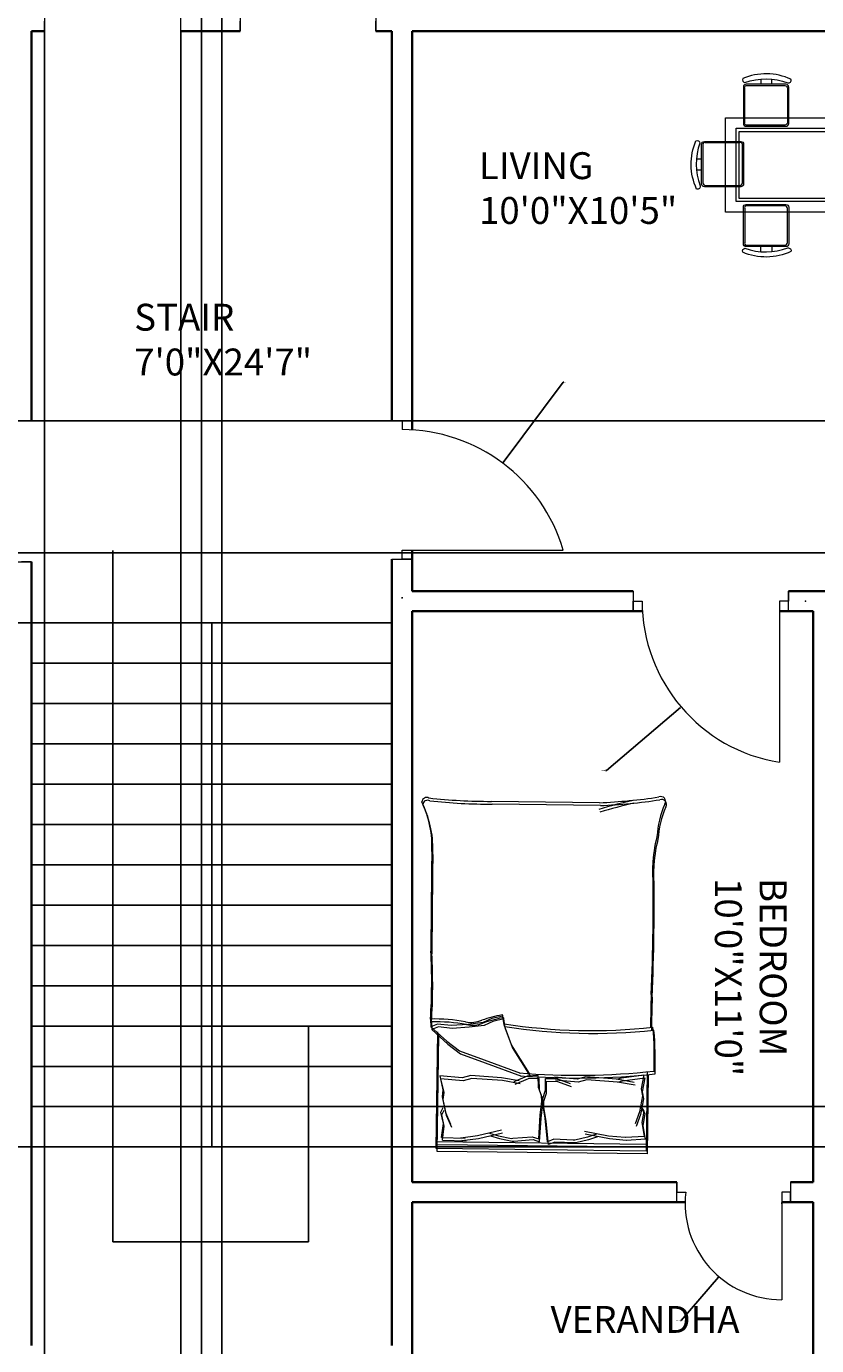
# Model space of a CAD drawing. Units: inches. Extents: x 1721 to 2510, y 1544 to 2360.
# Tile 4 of 10: x 2046 to 2222, y 1693 to 1988. Entities that reach past the tile are written whole.
import ezdxf

# ---------------------------------------------------------------- set-up
doc = ezdxf.new("R2010")
doc.units = ezdxf.units.IN
for name, color, linetype, lineweight in [('A-ANNO-DIMS', 2, 'Continuous', 18), ('A-AREA-IDEN', 7, 'Continuous', 18), ('A-DOOR', 3, 'Continuous', 18), ('A-FLOR-STRS', 7, 'Continuous', 25), ('A-FURN', 8, 'Continuous', 13), ('A-WALL', 7, 'Continuous', 35)]:
    doc.layers.add(name, color=color, linetype=linetype, lineweight=lineweight)
doc.styles.get("Standard").update_dxf_attribs({"font": 'arial.ttf'})
doc.dimstyles.get("Standard").update_dxf_attribs({"dimtxt": 0.18, "dimasz": 0.18, "dimexe": 0.18, "dimexo": 0.0625, "dimgap": 0.09, "dimtad": 0, "dimtih": 1, "dimtoh": 1, "dimdec": 4, "dimzin": 0, "dimdsep": 46, "dimtxsty": 'Standard', "dimcen": 0.09, "dimadec": 0, "dimazin": 0, "dimtfac": 1, "dimtdec": 4, "dimtofl": 0, "dimtmove": 0, "dimatfit": 3, "dimfxl": 1, "dimtolj": 1, "dimtzin": 0, "dimarcsym": 0})

# ---------------------------------------------------------------- blocks, each defined once
blk = doc.blocks.new('BED-DOUBLE')
for p, q in [((39.64, 78.43), (15.52, 78.72)), ((39.64, 78.43), (15.52, 78.72)), ((39.86, 77.8), (15.74, 78.09)), ((39.86, 77.8), (15.74, 78.09)), ((1.93, 30.11), (1.99, 28.4, 3.79)), ((1.93, 30.11), (1.99, 28.4, 3.79)), ((2.15, 29.48), (2.21, 27.77, 3.79)), ((2.15, 29.48), (2.21, 27.77, 3.79)), ((15.66, 30.21), (13.68, 29.32)), ((15.66, 30.21), (13.68, 29.32)), ((15.88, 29.58), (13.89, 28.69)), ((15.88, 29.58), (13.89, 28.69)), ((18.1, 30.79), (15.66, 30.21)), ((18.1, 30.79), (15.66, 30.21)), ((18.31, 30.16), (15.88, 29.58)), ((18.31, 30.16), (15.88, 29.58)), ((18.38, 28.81), (18.1, 30.79)), ((18.38, 28.81), (18.1, 30.79)), ((18.59, 28.18), (18.31, 30.16)), ((18.59, 28.18), (18.31, 30.16)), ((3.5, 28.99), (1.99, 28.4)), ((3.5, 28.99), (1.99, 28.4)), ((1.99, 28.4), (5.58, 25.17)), ((1.99, 28.4), (5.58, 25.17)), ((3.72, 28.36), (2.21, 27.77)), ((3.72, 28.36), (2.21, 27.77)), ((2.21, 27.77), (5.8, 24.54)), ((2.21, 27.77), (5.8, 24.54)), ((3.23, 1.19), (3.55, 27.27)), ((3.23, 1.19), (3.55, 27.27)), ((3.45, 0.56), (3.76, 26.64)), ((3.45, 0.56), (3.76, 26.64)), ((6.54, 28.65), (3.5, 28.99)), ((6.54, 28.65), (3.5, 28.99)), ((6.75, 28.02), (3.72, 28.36)), ((6.75, 28.02), (3.72, 28.36)), ((10.33, 28.91), (6.54, 28.65)), ((10.33, 28.91), (6.54, 28.65)), ((10.55, 28.28), (6.75, 28.02)), ((10.55, 28.28), (6.75, 28.02)), ((13.68, 29.32), (10.33, 28.91)), ((13.68, 29.32), (10.33, 28.91)), ((13.89, 28.69), (10.55, 28.28)), ((13.89, 28.69), (10.55, 28.28)), ((20, 24.39), (18.38, 28.81)), ((20, 24.39), (18.38, 28.81)), ((20.21, 23.76), (18.59, 28.18)), ((20.21, 23.76), (18.59, 28.18)), ((5.58, 25.17), (8.44, 23.01)), ((5.58, 25.17), (8.44, 23.01)), ((5.8, 24.54), (8.66, 22.38)), ((5.8, 24.54), (8.66, 22.38)), ((24.03, 17.98), (20, 24.39)), ((24.03, 17.98), (20, 24.39)), ((24.24, 17.35), (20.21, 23.76)), ((24.24, 17.35), (20.21, 23.76)), ((8.44, 23.01), (13.88, 20.98)), ((8.44, 23.01), (13.88, 20.98)), ((8.66, 22.38), (14.1, 20.35)), ((8.66, 22.38), (14.1, 20.35)), ((13.88, 20.98), (22.02, 18)), ((13.88, 20.98), (22.02, 18)), ((14.1, 20.35), (22.24, 17.37)), ((14.1, 20.35), (22.24, 17.37)), ((50.28, 18.38), (50.07, 0.63)), ((50.28, 18.38), (50.07, 0.63)), ((50.5, 17.75), (50.29, 0)), ((50.5, 17.75), (50.29, 0)), ((9.01, 16.97), (3.98, 17.42)), ((3.98, 17.42), (4.71, 14.34)), ((9.01, 16.97), (3.98, 17.42)), ((3.98, 17.42), (4.71, 14.34)), ((9.23, 16.34), (4.2, 16.8)), ((4.2, 16.8), (4.92, 13.71)), ((9.23, 16.34), (4.2, 16.8)), ((4.2, 16.8), (4.92, 13.71)), ((10.94, 17.49), (9.01, 16.97)), ((10.94, 17.49), (9.01, 16.97)), ((11.15, 16.86), (9.23, 16.34)), ((11.15, 16.86), (9.23, 16.34)), ((17.8, 16.99), (10.94, 17.49)), ((17.8, 16.99), (10.94, 17.49)), ((18.02, 16.36), (11.15, 16.86)), ((18.02, 16.36), (11.15, 16.86)), ((21.75, 16.29), (17.8, 16.99)), ((21.75, 16.29), (17.8, 16.99)), ((21.96, 15.66), (18.02, 16.36)), ((21.96, 15.66), (18.02, 16.36)), ((23.54, 17.35), (20.51, 16.13)), ((23.54, 17.35), (20.51, 16.13)), ((23.75, 16.73), (20.73, 15.5)), ((23.75, 16.73), (20.73, 15.5)), ((25.94, 17.48), (23.54, 17.35)), ((25.94, 17.48), (23.54, 17.35)), ((26.16, 16.85), (23.75, 16.73)), ((26.16, 16.85), (23.75, 16.73)), ((26.07, 14.85), (25.94, 17.48)), ((26.07, 14.85), (25.94, 17.48)), ((26.73, 13.04), (26.07, 14.85)), ((26.73, 13.04), (26.07, 14.85)), ((26.29, 14.22), (26.16, 16.85)), ((26.29, 14.22), (26.16, 16.85)), ((27.61, 14.21), (27.64, 16.84)), ((27.61, 14.21), (27.64, 16.84)), ((27.64, 16.84), (30.05, 16.81)), ((27.64, 16.84), (30.05, 16.81)), ((27.82, 13.58), (27.85, 16.21)), ((27.82, 13.58), (27.85, 16.21)), ((27.85, 16.21), (30.26, 16.18)), ((27.85, 16.21), (30.26, 16.18)), ((34.67, 16.66), (29.65, 17.12)), ((34.67, 16.66), (29.65, 17.12)), ((34.89, 16.03), (29.86, 16.49)), ((34.89, 16.03), (29.86, 16.49)), ((30.05, 16.81), (33.11, 15.7)), ((30.05, 16.81), (33.11, 15.7)), ((30.26, 16.18), (33.33, 15.07)), ((30.26, 16.18), (33.33, 15.07)), ((36.6, 17.19), (34.67, 16.66)), ((36.6, 17.19), (34.67, 16.66)), ((36.81, 16.56), (34.89, 16.03)), ((36.81, 16.56), (34.89, 16.03)), ((43.46, 16.68), (36.6, 17.19)), ((43.46, 16.68), (36.6, 17.19)), ((43.68, 16.05), (36.81, 16.56)), ((43.68, 16.05), (36.81, 16.56)), ((43.46, 16.68), (44.58, 16.98)), ((43.46, 16.68), (44.58, 16.98)), ((47.41, 15.98), (43.46, 16.68)), ((47.41, 15.98), (43.46, 16.68)), ((43.68, 16.05), (44.79, 16.35)), ((43.68, 16.05), (44.79, 16.35)), ((47.62, 15.35), (43.68, 16.05)), ((47.62, 15.35), (43.68, 16.05)), ((44.58, 16.98), (49.58, 17.63)), ((44.58, 16.98), (49.58, 17.63)), ((44.79, 16.35), (49.8, 17)), ((44.79, 16.35), (49.8, 17)), ((49.58, 17.63), (48.98, 14.52)), ((49.58, 17.63), (48.98, 14.52)), ((49.8, 17), (49.19, 13.89)), ((49.8, 17), (49.19, 13.89)), ((4.71, 14.34), (4.5, 12.77)), ((4.71, 14.34), (4.5, 12.77)), ((4.5, 12.77), (5.25, 9.26)), ((4.5, 12.77), (5.25, 9.26)), ((4.92, 13.71), (4.72, 12.14)), ((4.92, 13.71), (4.72, 12.14)), ((4.72, 12.14), (5.46, 8.63)), ((4.72, 12.14), (5.46, 8.63)), ((26.95, 12.41), (26.29, 14.22)), ((26.95, 12.41), (26.29, 14.22)), ((26.8, 11.77), (26.73, 13.04)), ((26.8, 11.77), (26.73, 13.04)), ((27.01, 11.14), (26.95, 12.41)), ((27.01, 11.14), (26.95, 12.41)), ((27, 11.1), (27.02, 12.38)), ((27, 11.1), (27.02, 12.38)), ((27.02, 12.38), (27.61, 14.21)), ((27.02, 12.38), (27.61, 14.21)), ((27.23, 11.75), (27.82, 13.58)), ((27.23, 11.75), (27.82, 13.58)), ((49.24, 12.96), (48.63, 9.42)), ((49.24, 12.96), (48.63, 9.42)), ((49.46, 12.33), (48.85, 8.79)), ((49.46, 12.33), (48.85, 8.79)), ((48.98, 14.52), (49.24, 12.96)), ((48.98, 14.52), (49.24, 12.96)), ((49.19, 13.89), (49.46, 12.33)), ((49.19, 13.89), (49.46, 12.33)), ((4.25, 9.35), (4.77, 10.37)), ((4.25, 9.35), (4.77, 10.37)), ((4.8, 6.82), (4.25, 9.35)), ((4.8, 6.82), (4.25, 9.35)), ((4.47, 8.72), (4.98, 9.74)), ((4.47, 8.72), (4.98, 9.74)), ((5.25, 9.26), (6.37, 6.62)), ((5.25, 9.26), (6.37, 6.62)), ((26.39, 8.62), (26.8, 11.77)), ((26.39, 8.62), (26.8, 11.77)), ((26.61, 7.99), (27.01, 11.14)), ((26.61, 7.99), (27.01, 11.14)), ((27.53, 7.98), (27, 11.1)), ((27.53, 7.98), (27, 11.1)), ((27.22, 10.47), (27.23, 11.75)), ((27.22, 10.47), (27.23, 11.75)), ((27.75, 7.35), (27.22, 10.47)), ((27.75, 7.35), (27.22, 10.47)), ((48.63, 9.42), (47.61, 6.74)), ((48.63, 9.42), (47.61, 6.74)), ((49.63, 9.55), (49.07, 10.55)), ((49.63, 9.55), (49.07, 10.55)), ((49.17, 7.01), (49.63, 9.55)), ((49.17, 7.01), (49.63, 9.55)), ((49.84, 8.92), (49.29, 9.92)), ((49.84, 8.92), (49.29, 9.92)), ((49.39, 6.38), (49.84, 8.92)), ((49.39, 6.38), (49.84, 8.92)), ((4.39, 3.68), (4.8, 6.82)), ((4.39, 3.68), (4.8, 6.82)), ((5.02, 6.19), (4.47, 8.72)), ((5.02, 6.19), (4.47, 8.72)), ((4.61, 3.05), (5.02, 6.19)), ((4.61, 3.05), (5.02, 6.19)), ((5.46, 8.63), (6.59, 5.99)), ((5.46, 8.63), (6.59, 5.99)), ((26.09, 3.36), (26.39, 8.62)), ((26.09, 3.36), (26.39, 8.62)), ((26.3, 2.73), (26.61, 7.99)), ((26.3, 2.73), (26.61, 7.99)), ((28.04, 2.73), (27.53, 7.98)), ((28.04, 2.73), (27.53, 7.98)), ((28.25, 2.1), (27.75, 7.35)), ((28.25, 2.1), (27.75, 7.35)), ((48.85, 8.79), (47.82, 6.11)), ((48.85, 8.79), (47.82, 6.11)), ((49.7, 3.88), (49.17, 7.01)), ((49.7, 3.88), (49.17, 7.01)), ((49.92, 3.25), (49.39, 6.38)), ((49.92, 3.25), (49.39, 6.38)), ((4.39, 3.68), (9.69, 3.52)), ((4.39, 3.68), (9.69, 3.52)), ((4.61, 3.05), (9.9, 2.89)), ((4.61, 3.05), (9.9, 2.89)), ((8.71, 3.62), (12.44, 4.09)), ((8.71, 3.62), (12.44, 4.09)), ((9.69, 3.52), (8.71, 3.62)), ((9.69, 3.52), (8.71, 3.62)), ((8.92, 2.99), (12.65, 3.46)), ((8.92, 2.99), (12.65, 3.46)), ((9.9, 2.89), (8.92, 2.99)), ((9.9, 2.89), (8.92, 2.99)), ((12.44, 4.09), (17.76, 5.35)), ((12.44, 4.09), (17.76, 5.35)), ((12.65, 3.46), (17.98, 4.72)), ((12.65, 3.46), (17.98, 4.72)), ((15.1, 4.65), (17.12, 4.04)), ((15.1, 4.65), (17.12, 4.04)), ((15.32, 4.02), (17.34, 3.41)), ((15.32, 4.02), (17.34, 3.41)), ((17.12, 4.04), (19.98, 3.48)), ((17.12, 4.04), (19.98, 3.48)), ((17.34, 3.41), (20.2, 2.85)), ((17.34, 3.41), (20.2, 2.85)), ((19.98, 3.48), (20.3, 3.49)), ((19.98, 3.48), (20.3, 3.49)), ((20.3, 3.49), (24.64, 3.85)), ((20.3, 3.49), (24.64, 3.85)), ((20.52, 2.86), (24.86, 3.22)), ((20.52, 2.86), (24.86, 3.22)), ((24.64, 3.85), (26.09, 3.36)), ((24.64, 3.85), (26.09, 3.36)), ((24.86, 3.22), (26.3, 2.73)), ((24.86, 3.22), (26.3, 2.73)), ((29.46, 3.28), (28.04, 2.73)), ((29.46, 3.28), (28.04, 2.73)), ((33.81, 3.08), (29.46, 3.28)), ((33.81, 3.08), (29.46, 3.28)), ((34.13, 3.08), (33.81, 3.08)), ((34.13, 3.08), (33.81, 3.08)), ((36.97, 3.75), (34.13, 3.08)), ((36.97, 3.75), (34.13, 3.08)), ((37.19, 3.12), (34.35, 2.45)), ((37.19, 3.12), (34.35, 2.45)), ((41.65, 3.98), (36.28, 5.04)), ((41.65, 3.98), (36.28, 5.04)), ((41.87, 3.35), (36.49, 4.41)), ((41.87, 3.35), (36.49, 4.41)), ((38.96, 4.44), (36.97, 3.75)), ((38.96, 4.44), (36.97, 3.75)), ((39.18, 3.81), (37.19, 3.12)), ((39.18, 3.81), (37.19, 3.12)), ((45.39, 3.65), (41.65, 3.98)), ((45.39, 3.65), (41.65, 3.98)), ((45.61, 3.02), (41.87, 3.35)), ((45.61, 3.02), (41.87, 3.35)), ((45.5, 3.63), (45.39, 3.65)), ((45.5, 3.63), (45.39, 3.65)), ((49.7, 3.91), (45.5, 3.63)), ((49.7, 3.91), (45.5, 3.63)), ((45.71, 3), (45.61, 3.02)), ((45.71, 3), (45.61, 3.02)), ((49.91, 3.28), (45.71, 3)), ((49.91, 3.28), (45.71, 3)), ((50.07, 0.63), (3.23, 1.19)), ((50.07, 0.63), (3.23, 1.19)), ((50.09, 2.13), (3.25, 2.69)), ((50.09, 2.13), (3.25, 2.69)), ((50.29, 0), (3.45, 0.56)), ((50.29, 0), (3.45, 0.56)), ((50.31, 1.5), (3.47, 2.06)), ((50.31, 1.5), (3.47, 2.06)), ((20.2, 2.85), (20.52, 2.86)), ((20.2, 2.85), (20.52, 2.86)), ((29.68, 2.65), (28.25, 2.1)), ((29.68, 2.65), (28.25, 2.1)), ((34.03, 2.45), (29.68, 2.65)), ((34.03, 2.45), (29.68, 2.65)), ((34.35, 2.45), (34.03, 2.45)), ((34.35, 2.45), (34.03, 2.45))]:
    blk.add_line(p, q)
for centre, radius, start, end in [((1.08, 78.52), 1.08, 61.9736, 175.3348), ((1.08, 78.52), 1.08, 61.9736, 175.3348), ((34.83, 197.67), 119.34, 272.3106, 278.7239), ((34.83, 197.67), 119.34, 272.3106, 278.7239), ((53.35, 78.73), 1.07, 325.4884, 112.793), ((53.35, 78.73), 1.07, 325.4884, 112.793), ((-20.36, 68.78), 22.61, 356.7862, 25.7829), ((-20.36, 68.78), 22.61, 356.7862, 25.7829), ((1.29, 77.89), 1.08, 61.9736, 175.3348), ((1.29, 77.89), 1.08, 61.9736, 175.3348), ((-20.14, 68.15), 22.61, 356.7862, 25.7829), ((-20.14, 68.15), 22.61, 356.7862, 25.7829), ((15.63, 209.12), 130.4, 263.8146, 269.9499), ((15.63, 209.12), 130.4, 263.8146, 269.9499), ((15.85, 208.49), 130.4, 263.8146, 269.9499), ((15.85, 208.49), 130.4, 263.8146, 269.9499), ((70.08, -22.85), 104.34, 102.698, 107.0202), ((70.08, -22.85), 104.34, 102.698, 107.0202), ((70.29, -23.48), 104.34, 102.698, 107.0202), ((70.29, -23.48), 104.34, 102.698, 107.0202), ((35.05, 197.04), 119.34, 272.3106, 278.7239), ((35.05, 197.04), 119.34, 272.3106, 278.7239), ((75.53, 69.21), 23.09, 157.2899, 175.9668), ((75.53, 69.21), 23.09, 157.2899, 175.9668), ((75.75, 68.58), 23.09, 157.2899, 175.9668), ((75.75, 68.58), 23.09, 157.2899, 175.9668), ((53.56, 78.1), 1.07, 325.4884, 112.793), ((53.56, 78.1), 1.07, 325.4884, 112.793), ((80.6, 63.5), 29.05, 165.3797, 178.2261), ((80.6, 63.5), 29.05, 165.3797, 178.2261), ((80.81, 62.87), 29.05, 165.3797, 178.2261), ((80.81, 62.87), 29.05, 165.3797, 178.2261), ((4473.12, 14.21), 4471.22, 179.317, 179.60172), ((4473.12, 14.21), 4471.22, 179.317, 179.60172), ((4473.34, 13.58), 4471.22, 179.317, 179.60172), ((4473.34, 13.58), 4471.22, 179.317, 179.60172), ((-421.08, 55.88), 472.73, 357.5425, 1.0334), ((-421.08, 55.88), 472.73, 357.5425, 1.0334), ((-420.87, 55.25), 472.73, 357.5425, 1.0334), ((-420.87, 55.25), 472.73, 357.5425, 1.0334), ((-124.73, 38.32), 126.93, 356.294, 3.1513), ((-124.73, 38.32), 126.93, 356.294, 3.1513), ((-124.51, 37.69), 126.93, 356.294, 3.1513), ((-124.51, 37.69), 126.93, 356.294, 3.1513), ((217.81, 29.18), 166.73, 177.791, 180.323), ((217.81, 29.18), 166.73, 177.791, 180.323), ((218.03, 28.55), 166.73, 177.791, 180.323), ((218.03, 28.55), 166.73, 177.791, 180.323), ((3.1, -5.33), 35.46, 79.1911, 91.8805), ((3.1, -5.33), 35.46, 79.1911, 91.8805), ((3.31, -5.96), 35.46, 79.1911, 91.8805), ((3.31, -5.96), 35.46, 79.1911, 91.8805), ((11.02, 35.47), 6.1, 257.9756, 293.0532), ((11.02, 35.47), 6.1, 257.9756, 293.0532), ((22.96, 2.41), 29.06, 99.9765, 109.1954), ((22.96, 2.41), 29.06, 99.9765, 109.1954), ((23.18, 1.78), 29.06, 99.9765, 109.1954), ((23.18, 1.78), 29.06, 99.9765, 109.1954), ((17.93, 30.85), 0.181, 339.5612, 90.4525), ((17.93, 30.85), 0.181, 339.5612, 90.4525), ((18.15, 30.22), 0.181, 339.5612, 90.4525), ((18.15, 30.22), 0.181, 339.5612, 90.4525), ((11.23, 34.84), 6.1, 257.9756, 293.0532), ((11.23, 34.84), 6.1, 257.9756, 293.0532), ((37.91, 154), 126.46, 261.0993, 276.2154), ((37.91, 154), 126.46, 261.0993, 276.2154), ((38.12, 153.37), 126.46, 261.0993, 276.2154), ((38.12, 153.37), 126.46, 261.0993, 276.2154), ((-29.75, 21.28), 81.65, 358.0366, 4.9188), ((-29.75, 21.28), 81.65, 358.0366, 4.9188), ((-29.53, 20.65), 81.65, 358.0366, 4.9188), ((-29.53, 20.65), 81.65, 358.0366, 4.9188), ((34.68, 179.26), 161.69, 265.4014, 276.097), ((34.68, 179.26), 161.69, 265.4014, 276.097), ((34.89, 178.63), 161.69, 265.4014, 276.097), ((34.89, 178.63), 161.69, 265.4014, 276.097)]:
    blk.add_arc(centre, radius, start, end)
blk = doc.blocks.new('TABLE-DINING-RECT')
for points in [[(0, 21.04), (35.07, 21.04), (35.07, 0), (0, 0)], [(2.34, 18.71), (32.73, 18.71), (32.73, 2.34), (2.34, 2.34)], [(3.04, 18), (32.03, 18), (32.03, 3.04), (3.04, 3.04)]]:
    blk.add_lwpolyline(points, close=True)
blk = doc.blocks.new('CHAIR-DINING-A')
for points in [[(2.02, 0.75, -0.578392), (1.23, 0.03, -0.214524), (1.08, 10.81, -0.552014), (1.95, 10.31, 0.175809), (2.02, 0.75)], [(2.34, 10.03, -0.414214), (2.96, 10.65), (11.11, 10.65, -0.414214), (11.73, 10.03), (11.73, 1.16, -0.414214), (11.11, 0.54), (2.96, 0.54, -0.414214), (2.34, 1.16), (2.34, 10.03)], [(2.34, 4.27), (1.21, 4.27, 0.064759)]]:
    blk.add_lwpolyline(points, format="xyb")
blk.add_lwpolyline([(2.62, 10.02), (2.62, 1.44, 0.414214), (3.24, 0.82), (10.83, 0.82, 0.414214), (11.45, 1.44), (11.45, 10.02, 0.512069), (10.83, 10.37), (3.24, 10.37, 0.512069)], format="xyb", close=True)
blk.add_lwpolyline([(1.19, 6.76), (2.34, 6.76)])
blk = doc.blocks.new('*D53')
at = {"layer": 'A-ANNO-DIMS', "color": 0, "lineweight": -2, "transparency": 16777216}
for p, q in [((2127.44, 1854.49), (1765.42, 1854.49)), ((1765.6, 1854.31), (1765.6, 1796.17)), ((1765.6, 1737.67), (1765.6, 1795.81)), ((2127.44, 1737.49), (1765.42, 1737.49))]:
    blk.add_line(p, q, dxfattribs=at)
at = {"layer": 'A-ANNO-DIMS', "color": 0, "transparency": 16777216}
for points in [[(1765.57, 1854.31), (1765.63, 1854.31), (1765.6, 1854.49)], [(1765.57, 1737.67), (1765.63, 1737.67), (1765.6, 1737.49)]]:
    blk.add_solid(points, dxfattribs=at)
at = {"layer": 'Defpoints', "color": 0, "transparency": 16777216}
for p in [(1765.6, 1854.49), (2127.5, 1854.49), (2127.5, 1737.49)]:
    blk.add_point(p, dxfattribs=at)
at = {"layer": 'A-ANNO-DIMS', "color": 0, "transparency": 16777216, "insert": (1765.6, 1795.99), "char_height": 0.18, "attachment_point": 5}
blk.add_mtext('\\A1;117', dxfattribs=at)
blk = doc.blocks.new('*D54')
at = {"layer": 'A-ANNO-DIMS', "color": 0, "lineweight": -2, "transparency": 16777216}
for p, q in [((2047.06, 1746.49), (2409.08, 1746.49)), ((2408.9, 1746.31), (2408.9, 1742.17)), ((2408.9, 1737.67), (2408.9, 1741.81)), ((2047.06, 1737.49), (2409.08, 1737.49))]:
    blk.add_line(p, q, dxfattribs=at)
at = {"layer": 'A-ANNO-DIMS', "color": 0, "transparency": 16777216}
for points in [[(2408.87, 1746.31), (2408.93, 1746.31), (2408.9, 1746.49)], [(2408.87, 1737.67), (2408.93, 1737.67), (2408.9, 1737.49)]]:
    blk.add_solid(points, dxfattribs=at)
at = {"layer": 'Defpoints', "color": 0, "transparency": 16777216}
for p in [(2047, 1746.49), (2408.9, 1746.49), (2047, 1737.49)]:
    blk.add_point(p, dxfattribs=at)
at = {"layer": 'A-ANNO-DIMS', "color": 0, "transparency": 16777216, "insert": (2408.9, 1741.99), "char_height": 0.18, "attachment_point": 5}
blk.add_mtext('\\A1;9', dxfattribs=at)
blk = doc.blocks.new('*D58')
at = {"layer": 'A-ANNO-DIMS', "color": 0, "lineweight": -2, "transparency": 16777216}
for p, q in [((2042.56, 1899.66), (2409.08, 1899.66)), ((2408.9, 1899.48), (2408.9, 1885.09)), ((2408.9, 1870.34), (2408.9, 1884.73)), ((2042.56, 1870.16), (2409.08, 1870.16))]:
    blk.add_line(p, q, dxfattribs=at)
at = {"layer": 'A-ANNO-DIMS', "color": 0, "transparency": 16777216}
for points in [[(2408.87, 1899.48), (2408.93, 1899.48), (2408.9, 1899.66)], [(2408.87, 1870.34), (2408.93, 1870.34), (2408.9, 1870.16)]]:
    blk.add_solid(points, dxfattribs=at)
at = {"layer": 'Defpoints', "color": 0, "transparency": 16777216}
for p in [(2042.5, 1899.66), (2408.9, 1899.66), (2042.5, 1870.16)]:
    blk.add_point(p, dxfattribs=at)
at = {"layer": 'A-ANNO-DIMS', "color": 0, "transparency": 16777216, "insert": (2408.9, 1884.91), "char_height": 0.18, "attachment_point": 5}
blk.add_mtext('\\A1;29.505', dxfattribs=at)
blk = doc.blocks.new('*D64')
at = {"layer": 'A-ANNO-DIMS', "color": 0, "lineweight": -2, "transparency": 16777216}
for p, q in [((2049.89, 1986.57), (2049.89, 1606.75)), ((2080.39, 1986.57), (2080.39, 1606.75)), ((2050.07, 1606.93), (2064.81, 1606.93)), ((2080.21, 1606.93), (2065.46, 1606.93))]:
    blk.add_line(p, q, dxfattribs=at)
at = {"layer": 'A-ANNO-DIMS', "color": 0, "transparency": 16777216}
for points in [[(2050.07, 1606.96), (2050.07, 1606.9), (2049.89, 1606.93)], [(2080.21, 1606.96), (2080.21, 1606.9), (2080.39, 1606.93)]]:
    blk.add_solid(points, dxfattribs=at)
at = {"layer": 'Defpoints', "color": 0, "transparency": 16777216}
for p in [(2049.89, 1986.63), (2080.39, 1986.63), (2080.39, 1606.93)]:
    blk.add_point(p, dxfattribs=at)
at = {"layer": 'A-ANNO-DIMS', "color": 0, "transparency": 16777216, "insert": (2065.14, 1606.93), "char_height": 0.18, "attachment_point": 5}
blk.add_mtext('\\A1;30.5', dxfattribs=at)
blk = doc.blocks.new('*D65')
at = {"layer": 'A-ANNO-DIMS', "color": 0, "lineweight": -2, "transparency": 16777216}
for p, q in [((2085, 2116.38), (2085, 1606.75)), ((2089.5, 2116.38), (2089.5, 1606.75)), ((2085.18, 1606.93), (2086.99, 1606.93)), ((2089.32, 1606.93), (2087.51, 1606.93))]:
    blk.add_line(p, q, dxfattribs=at)
at = {"layer": 'A-ANNO-DIMS', "color": 0, "transparency": 16777216}
for points in [[(2085.18, 1606.96), (2085.18, 1606.9), (2085, 1606.93)], [(2089.32, 1606.96), (2089.32, 1606.9), (2089.5, 1606.93)]]:
    blk.add_solid(points, dxfattribs=at)
at = {"layer": 'Defpoints', "color": 0, "transparency": 16777216}
for p in [(2085, 2116.44), (2089.5, 2116.44), (2089.5, 1606.93)]:
    blk.add_point(p, dxfattribs=at)
at = {"layer": 'A-ANNO-DIMS', "color": 0, "transparency": 16777216, "insert": (2087.25, 1606.93), "char_height": 0.18, "attachment_point": 5}
blk.add_mtext('\\A1;4.5', dxfattribs=at)
blk = doc.blocks.new('*D69')
at = {"layer": 'A-ANNO-DIMS', "color": 0, "lineweight": -2, "transparency": 16777216}
for p, q in [((2165.71, 1908.23), (2152.33, 1890.34)), ((2165.89, 1908.23), (2165.71, 1908.23)), ((2129.66, 1860.13), (2129.84, 1860.13)), ((2129.75, 1860.04), (2129.75, 1860.22))]:
    blk.add_line(p, q, dxfattribs=at)
at = {"layer": 'A-ANNO-DIMS', "color": 0, "transparency": 16777216}
blk.add_solid([(2152.31, 1890.36), (2152.36, 1890.32), (2152.23, 1890.19)], dxfattribs=at)
at = {"layer": 'Defpoints', "color": 0, "transparency": 16777216}
for p in [(2152.23, 1890.19), (2129.75, 1860.13)]:
    blk.add_point(p, dxfattribs=at)
at = {"layer": 'A-ANNO-DIMS', "color": 0, "transparency": 16777216, "insert": (2166.44, 1908.23), "char_height": 0.18, "attachment_point": 5}
blk.add_mtext('\\A1;R37.536', dxfattribs=at)
blk = doc.blocks.new('*D71')
at = {"layer": 'A-ANNO-DIMS', "color": 0, "lineweight": -2, "transparency": 16777216}
for p, q in [((2219.72, 1859.38), (2219.9, 1859.38)), ((2219.81, 1859.29), (2219.81, 1859.47)), ((2175.39, 1821.55), (2191.91, 1835.62)), ((2175.21, 1821.55), (2175.39, 1821.55))]:
    blk.add_line(p, q, dxfattribs=at)
at = {"layer": 'A-ANNO-DIMS', "color": 0, "transparency": 16777216}
blk.add_solid([(2191.89, 1835.64), (2191.93, 1835.6), (2192.05, 1835.74)], dxfattribs=at)
at = {"layer": 'Defpoints', "color": 0, "transparency": 16777216}
for p in [(2219.81, 1859.38), (2192.05, 1835.74)]:
    blk.add_point(p, dxfattribs=at)
at = {"layer": 'A-ANNO-DIMS', "color": 0, "transparency": 16777216, "insert": (2174.66, 1821.55), "char_height": 0.18, "attachment_point": 5}
blk.add_mtext('\\A1;R36.465', dxfattribs=at)
blk = doc.blocks.new('*D95')
at = {"layer": 'A-ANNO-DIMS', "color": 0, "lineweight": -2, "transparency": 16777216}
for p, q in [((2214.42, 1724.93), (2214.6, 1724.93)), ((2214.51, 1724.84), (2214.51, 1725.02)), ((2192.07, 1698.75), (2200.37, 1708.43)), ((2191.89, 1698.75), (2192.07, 1698.75))]:
    blk.add_line(p, q, dxfattribs=at)
at = {"layer": 'A-ANNO-DIMS', "color": 0, "transparency": 16777216}
blk.add_solid([(2200.34, 1708.45), (2200.39, 1708.41), (2200.48, 1708.57)], dxfattribs=at)
at = {"layer": 'Defpoints', "color": 0, "transparency": 16777216}
for p in [(2214.51, 1724.93), (2200.48, 1708.57)]:
    blk.add_point(p, dxfattribs=at)
at = {"layer": 'A-ANNO-DIMS', "color": 0, "transparency": 16777216, "insert": (2191.34, 1698.75), "char_height": 0.18, "attachment_point": 5}
blk.add_mtext('\\A1;R21.553', dxfattribs=at)

msp = doc.modelspace()

# ---------------------------------------------------------------- linework, layer by layer
at = {"layer": 'A-DOOR'}
for p, q in [((2049.8856, 1991.1298), (2049.8856, 1986.6298)), ((2049.8856, 1986.6298), (2049.8856, 1988.8798)), ((2080.3854, 1986.6298), (2080.3854, 1991.1298)), ((2093.6307, 1991.1298), (2093.6307, 1986.6298)), ((2093.6307, 1986.6298), (2093.6307, 1988.8798)), ((2123.8777, 1991.1298), (2123.8777, 1986.6298)), ((2123.8777, 1986.6298), (2123.8777, 1988.8798)), ((2042.5024, 1899.6648), (2047.0024, 1899.6648)), ((2047.0024, 1899.6648), (2044.7524, 1899.6648)), ((2127.5024, 1899.6648), (2132.0024, 1899.6648)), ((2132.0024, 1899.6648), (2129.7524, 1899.6648)), ((2129.7524, 1899.6648), (2129.7524, 1897.6648)), ((2129.7524, 1868.7562), (2129.7524, 1870.7562)), ((2129.7524, 1870.7562), (2165.7524, 1870.7562)), ((2042.5024, 1868.1595), (2047.0024, 1868.1595)), ((2047.0024, 1868.1595), (2044.7524, 1868.1595)), ((2127.5024, 1868.7562), (2132.0024, 1868.7562)), ((2132.0024, 1868.7562), (2129.7524, 1868.7562)), ((2181.3474, 1861.6298), (2181.3474, 1857.1298)), ((2181.3474, 1857.1298), (2181.3474, 1859.3798)), ((2181.3474, 1859.3798), (2183.3474, 1859.3798)), ((2216.0057, 1859.3798), (2214.0057, 1859.3798)), ((2214.0057, 1859.3798), (2214.0057, 1823.3798)), ((2216.0057, 1857.1298), (2216.0057, 1861.6298)), ((2216.0057, 1861.6298), (2216.0057, 1859.3798)), ((2191.0943, 1725.1298), (2191.0943, 1729.6298)), ((2191.0943, 1729.6298), (2191.0943, 1727.3798)), ((2216.5084, 1729.6298), (2216.5084, 1725.1298)), ((2191.0943, 1727.3798), (2193.0943, 1727.3798)), ((2216.5084, 1727.3798), (2214.5084, 1727.3798)), ((2214.5084, 1727.3798), (2214.5084, 1703.3798)), ((2216.5084, 1725.1298), (2216.5084, 1727.3798))]:
    msp.add_line(p, q, dxfattribs=at)
for centre, radius, start, end in [((2129.7524, 1860.1289), 37.5358, 16.44669, 90), ((2219.8128, 1859.3798), 36.4654, 180, 260.836699), ((2214.5084, 1724.9333), 21.5535, 173.482354, 270)]:
    msp.add_arc(centre, radius, start, end, dxfattribs=at)
at = {"layer": 'A-FLOR-STRS'}
for p, q in [((2065.1933, 1870.6662), (2065.1933, 1716.3329)), ((2047.0024, 1854.4881), (2127.5024, 1854.4881)), ((2127.5024, 1854.4881), (2087.2524, 1854.4881)), ((2087.2524, 1854.4881), (2087.2524, 1737.4881)), ((2127.5024, 1854.4881), (2127.5024, 1854.4881)), ((2047.0024, 1845.4881), (2127.5024, 1845.4881)), ((2047.0024, 1836.4881), (2127.5024, 1836.4881)), ((2047.0024, 1827.4881), (2127.5024, 1827.4881)), ((2047.0024, 1818.4881), (2127.5024, 1818.4881)), ((2047.0024, 1809.4881), (2127.5024, 1809.4881)), ((2047.0024, 1800.4881), (2127.5024, 1800.4881)), ((2047.0024, 1791.4881), (2127.5024, 1791.4881)), ((2047.0024, 1782.4881), (2127.5024, 1782.4881)), ((2047.0024, 1773.4881), (2127.5024, 1773.4881)), ((2047.0024, 1764.4881), (2127.5024, 1764.4881)), ((2108.8802, 1716.3329), (2108.8802, 1764.4881)), ((2047.0024, 1755.4881), (2127.5024, 1755.4881)), ((2047.0024, 1746.4881), (2127.5024, 1746.4881)), ((2047.0024, 1737.4881), (2127.5024, 1737.4881)), ((2065.1933, 1716.3329), (2108.8802, 1716.3329))]:
    msp.add_line(p, q, dxfattribs=at)
at = {"layer": 'A-FURN'}
for points in [[(2206.3105, 1975.1734, -0.17580919), (2215.8634, 1975.1011, 0.57839206), (2216.5871, 1975.8968, 0.21452438), (2205.8039, 1976.0415, 0.55201397), (2206.3105, 1975.1734, -0.06507904)], [(2215.4581, 1974.79), (2206.5896, 1974.79, 0.41421356), (2205.9691, 1974.1696), (2205.9691, 1966.0151, 0.41421356), (2206.5896, 1965.3946), (2215.4581, 1965.3946, 0.41421356), (2216.0786, 1966.0151), (2216.0786, 1974.1696, 0.41421356), (2215.4581, 1974.79)], [(2212.343, 1974.79), (2212.343, 1975.9116, -0.06475861)], [(2215.4581, 1938.5415), (2206.5896, 1938.5415, -0.41421356), (2205.9691, 1939.1619), (2205.9691, 1947.3164, -0.41421356), (2206.5896, 1947.9368), (2215.4581, 1947.9368, -0.41421356), (2216.0786, 1947.3164), (2216.0786, 1939.1619, -0.41421356), (2215.4581, 1938.5415)], [(2212.343, 1938.5415), (2212.343, 1937.4199, 0.06475861)], [(2215.8634, 1938.2304, -0.57839206), (2216.5871, 1937.4346, -0.21452438), (2205.8039, 1937.29, -0.55201397), (2206.3105, 1938.1581, 0.17580929), (2215.8634, 1938.2304)]]:
    msp.add_lwpolyline(points, format="xyb", dxfattribs=at)
for points in [[(2206.5933, 1974.5105), (2215.1786, 1974.5105, -0.41421356), (2215.799, 1973.89), (2215.799, 1966.2946, -0.41421356), (2215.1786, 1965.6742), (2206.5933, 1965.6742, -0.51206948), (2206.2486, 1966.2946), (2206.2486, 1973.89, -0.51206948)], [(2206.5933, 1938.821), (2215.1786, 1938.821, 0.41421356), (2215.799, 1939.4414), (2215.799, 1947.0369, 0.41421356), (2215.1786, 1947.6573), (2206.5933, 1947.6573, 0.51206948), (2206.2486, 1947.0369), (2206.2486, 1939.4414, 0.51206948)]]:
    msp.add_lwpolyline(points, format="xyb", close=True, dxfattribs=at)
for points in [[(2209.8606, 1975.932), (2209.8606, 1974.79)], [(2209.8606, 1937.3995), (2209.8606, 1938.5415)]]:
    msp.add_lwpolyline(points, dxfattribs=at)
at = {"layer": 'A-WALL'}
for p, q in [((2047.0024, 1986.6298), (2047.0024, 1899.6648)), ((2047.0024, 1986.6298), (2049.8856, 1986.6298)), ((2080.3854, 1986.6298), (2093.6307, 1986.6298)), ((2123.8777, 1986.6298), (2127.5024, 1986.6298)), ((2127.5024, 1986.6298), (2127.5024, 1899.6648)), ((2247.5024, 1986.6298), (2132.0024, 1986.6298)), ((2132.0024, 1986.6298), (2132.0024, 1897.5973)), ((2132.0024, 1986.6298), (2247.5024, 1986.6298)), ((2132.0024, 1870.7562), (2132.0024, 1861.6298)), ((2047.0024, 1868.1595), (2047.0024, 1693.1298)), ((2127.5024, 1868.7562), (2127.5024, 1693.1298)), ((2181.3474, 1861.6298), (2132.0024, 1861.6298)), ((2231.5043, 1861.6298), (2216.0057, 1861.6298)), ((2132.0024, 1857.1298), (2183.4169, 1857.1298)), ((2132.0024, 1857.1298), (2132.0024, 1729.6298)), ((2214.0057, 1857.1298), (2221.5024, 1857.1298)), ((2221.5024, 1857.1298), (2221.5024, 1729.6298)), ((2191.0943, 1729.6298), (2132.0024, 1729.6298)), ((2221.5024, 1729.6298), (2216.5084, 1729.6298)), ((2132.0024, 1725.1298), (2192.9558, 1725.1298)), ((2132.0024, 1725.1298), (2132.0024, 1688.6298)), ((2214.5084, 1725.1298), (2221.5024, 1725.1298)), ((2221.5024, 1725.1298), (2221.5024, 1688.6298))]:
    msp.add_line(p, q, dxfattribs=at)

# ---------------------------------------------------------------- block references
at = {"layer": 'A-FURN'}
for name, p in [('TABLE-DINING-RECT', (2201.9727, 1946.2562)), ('CHAIR-DINING-A', (2194.2917, 1951.3522)), ('BED-DOUBLE', (2134.1707, 1735.9345))]:
    msp.add_blockref(name, p, dxfattribs=at)

# ---------------------------------------------------------------- texts
at = {"layer": 'A-AREA-IDEN', "char_height": 6, "attachment_point": 1}
for s, width, insert in [('LIVING\\P10\'0"X10\'5"', 100.575007, (2146.9274, 1959.6057)), ('STAIR\\P7\'0"X24\'7"', 95.052932, (2069.9513, 1925.7662)), ('VERANDHA', 91.048615, (2162.9099, 1701.9757))]:
    msp.add_mtext_dynamic_manual_height_columns(s, width=width, gutter_width=12.5, heights=[0], dxfattribs=dict(at, insert=insert))
at = {"layer": 'A-AREA-IDEN', "insert": (2215.6051, 1797.5407), "char_height": 6, "attachment_point": 1, "rotation": 270}
msp.add_mtext_dynamic_manual_height_columns('BEDROOM\\P10\'0"X11\'0"', width=68.113577, gutter_width=12.5, heights=[0], dxfattribs=at)

# ---------------------------------------------------------------- dimensions: what is measured, and where the dimension line sits
at = {"layer": 'A-ANNO-DIMS'}
for base, p1, p2, picture, middle in [((2089.5024, 1606.9297), (2085.0024, 2116.4416), (2089.5024, 2116.4416), '*D65', (2087.2524, 1606.9297)), ((2080.3854, 1606.9297), (2049.8856, 1986.6298), (2080.3854, 1986.6298), '*D64', (2065.1355, 1606.9297))]:
    dim = msp.add_linear_dim(base=base, p1=p1, p2=p2, dimstyle='Standard', override={"dimdec": 1, "dimlfac": 1, "dimrnd": 0, "dimzin": 0, "dimdsep": 46, "dimlunit": 2}, dxfattribs=at)
    dim.commit()
    dim.dimension.update_dxf_attribs({"geometry": picture, "text_midpoint": middle})
for center, mpoint, picture, middle in [((2129.7524, 1860.1289), (2152.2251, 1890.1941), '*D69', (2166.4384, 1908.2333)), ((2219.8128, 1859.3798), (2192.0508, 1835.7368), '*D71', (2174.6631, 1821.551)), ((2214.5084, 1724.9333), (2200.4849, 1708.5659), '*D95', (2191.3409, 1698.7455))]:
    dim = msp.add_radius_dim(center=center, mpoint=mpoint, dimstyle='Standard', override={"dimdec": 3, "dimlfac": 1, "dimrnd": 0, "dimzin": 0, "dimdsep": 46, "dimlunit": 2}, dxfattribs=at)
    dim.commit()
    dim.dimension.update_dxf_attribs({"geometry": picture, "text_midpoint": middle, "dimtype": 164})
for base, p1, p2, override, picture, middle in [((2408.9024, 1899.6648), (2042.5024, 1870.1595), (2042.5024, 1899.6648), {"dimdec": 3, "dimlfac": 1, "dimrnd": 0, "dimzin": 0, "dimdsep": 46, "dimlunit": 2}, '*D58', (2408.9024, 1884.9121)), ((1765.6024, 1854.4881), (2127.5024, 1737.4881), (2127.5024, 1854.4881), {"dimdec": 0, "dimlfac": 1, "dimrnd": 0, "dimzin": 0, "dimdsep": 46, "dimlunit": 2}, '*D53', (1765.6024, 1795.9881)), ((2408.9024, 1746.4881), (2047.0024, 1737.4881), (2047.0024, 1746.4881), {"dimdec": 0, "dimlfac": 1, "dimrnd": 0, "dimzin": 0, "dimdsep": 46, "dimlunit": 2}, '*D54', (2408.9024, 1741.9881))]:
    dim = msp.add_linear_dim(base=base, p1=p1, p2=p2, angle=90, dimstyle='Standard', override=override, dxfattribs=at)
    dim.commit()
    dim.dimension.update_dxf_attribs({"geometry": picture, "text_midpoint": middle})

doc.saveas('drawing.dxf')
